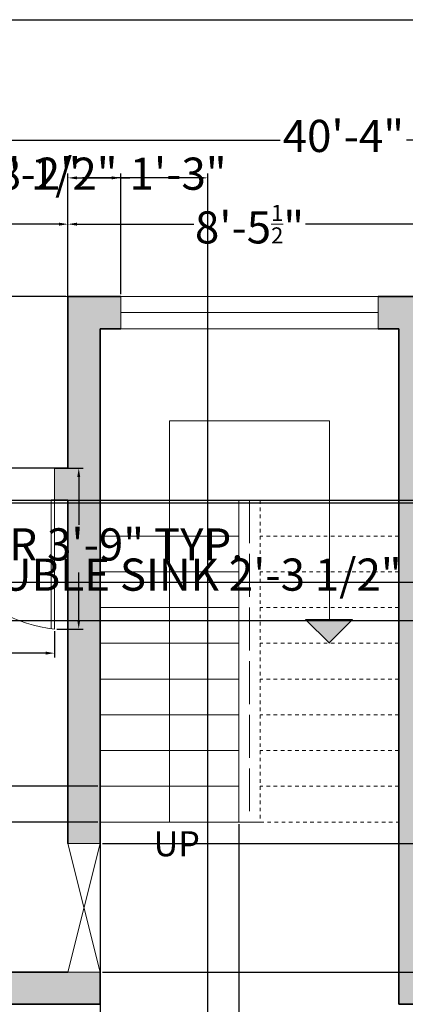
# Model space of a CAD drawing. Units: inches. Extents: x 1942 to 2601, y 2026 to 2623.
# Tile 3 of 5: x 2151 to 2259, y 2348 to 2623. Entities that reach past the tile are written whole.
import ezdxf

# ---------------------------------------------------------------- set-up
doc = ezdxf.new("R2010")
doc.units = ezdxf.units.IN
doc.linetypes.add('ACAD_ISO02W100', pattern=[15, 12, -3])
doc.linetypes.add('JIS_02_1.0', pattern=[2, 1, -1])
for name, color, linetype, lineweight in [('A-ANNO-DIMS', 2, 'Continuous', 18), ('A-ANNO-SYMB', 7, 'Continuous', 18), ('A-ANNO-TEXT', 7, 'Continuous', 18), ('A-ANNO-TTLB', 7, 'Continuous', 25), ('A-DOOR', 4, 'Continuous', 18), ('A-FLOR-OTLN', 8, 'ACAD_ISO02W100', 13), ('A-FLOR-STRS', 7, 'Continuous', 18), ('A-FLOR-STRS-CL', 8, 'ACAD_ISO02W100', 13), ('A-FLOR-STRS-HIDN', 7, 'JIS_02_1.0', 13), ('A-GLAZ', 2, 'Continuous', 18), ('A-WALL', 7, 'Continuous', 35), ('A-WALL-PATT', 7, 'Continuous', 13)]:
    doc.layers.add(name, color=color, linetype=linetype, lineweight=lineweight)
doc.styles.get("Standard").update_dxf_attribs({"font": 'arial.ttf'})
doc.dimstyles.new('ISO-25', dxfattribs={"dimtxt": 9, "dimasz": 2.5, "dimexe": 1.25, "dimexo": 0.625, "dimgap": 2, "dimtad": 0, "dimtih": 1, "dimtoh": 1, "dimdec": 1, "dimlunit": 4, "dimtxsty": 'Standard', "dimcen": 2.5, "dimadec": 0, "dimazin": 0, "dimtfac": 0.5, "dimtdec": 1, "dimtmove": 0, "dimatfit": 3, "dimfxl": 1, "dimarcsym": 0})

# ---------------------------------------------------------------- blocks, each defined once
blk = doc.blocks.new('*D11')
at = {"layer": 'A-ANNO-DIMS', "color": 0, "lineweight": -2, "transparency": 16777216}
for p, q in [((2164.82, 2546.54), (2164.82, 2567.42)), ((2266.32, 2546.54), (2266.32, 2567.42)), ((2167.32, 2566.17), (2199.96, 2566.17)), ((2263.82, 2566.17), (2231.18, 2566.17))]:
    blk.add_line(p, q, dxfattribs=at)
at = {"layer": 'A-ANNO-DIMS', "color": 0, "transparency": 16777216}
for points in [[(2167.32, 2566.58), (2167.32, 2565.75), (2164.82, 2566.17)], [(2263.82, 2566.58), (2263.82, 2565.75), (2266.32, 2566.17)]]:
    blk.add_solid(points, dxfattribs=at)
at = {"layer": 'Defpoints', "color": 0, "transparency": 16777216}
for p in [(2266.32, 2566.17), (2164.82, 2545.91), (2266.32, 2545.91)]:
    blk.add_point(p, dxfattribs=at)
at = {"layer": 'A-ANNO-DIMS', "color": 0, "transparency": 16777216, "insert": (2215.57, 2566.17), "char_height": 9, "attachment_point": 5}
blk.add_mtext('8\'-5{\\H0.5x;\\S1/2;}"', dxfattribs=at)
blk = doc.blocks.new('*D12')
at = {"layer": 'A-ANNO-DIMS', "color": 0, "lineweight": -2, "transparency": 16777216}
for p, q in [((1999.82, 2498.54), (1999.82, 2567.42)), ((2164.82, 2498.54), (2164.82, 2567.42)), ((2002.32, 2566.17), (2065.28, 2566.17)), ((2162.32, 2566.17), (2099.35, 2566.17))]:
    blk.add_line(p, q, dxfattribs=at)
at = {"layer": 'A-ANNO-DIMS', "color": 0, "transparency": 16777216}
for points in [[(2002.32, 2566.58), (2002.32, 2565.75), (1999.82, 2566.17)], [(2162.32, 2566.58), (2162.32, 2565.75), (2164.82, 2566.17)]]:
    blk.add_solid(points, dxfattribs=at)
at = {"layer": 'Defpoints', "color": 0, "transparency": 16777216}
for p in [(2164.82, 2566.17), (1999.82, 2497.91), (2164.82, 2497.91)]:
    blk.add_point(p, dxfattribs=at)
at = {"layer": 'A-ANNO-DIMS', "color": 0, "transparency": 16777216, "insert": (2082.32, 2566.17), "char_height": 9, "attachment_point": 5}
blk.add_mtext('13\'-9"', dxfattribs=at)
blk = doc.blocks.new('*D14')
at = {"layer": 'A-ANNO-DIMS', "color": 0, "lineweight": -2, "transparency": 16777216}
for p, q in [((1999.82, 2498.54), (1999.82, 2590.94)), ((2002.32, 2589.69), (2224.18, 2589.69)), ((2481.32, 2589.69), (2259.46, 2589.69)), ((2483.82, 2498.54), (2483.82, 2590.94))]:
    blk.add_line(p, q, dxfattribs=at)
at = {"layer": 'A-ANNO-DIMS', "color": 0, "transparency": 16777216}
for points in [[(2002.32, 2590.1), (2002.32, 2589.27), (1999.82, 2589.69)], [(2481.32, 2590.1), (2481.32, 2589.27), (2483.82, 2589.69)]]:
    blk.add_solid(points, dxfattribs=at)
at = {"layer": 'Defpoints', "color": 0, "transparency": 16777216}
for p in [(2483.82, 2589.69), (1999.82, 2497.91), (2483.82, 2497.91)]:
    blk.add_point(p, dxfattribs=at)
at = {"layer": 'A-ANNO-DIMS', "color": 0, "transparency": 16777216, "insert": (2241.82, 2589.69), "char_height": 9, "attachment_point": 5}
blk.add_mtext('40\'-4"', dxfattribs=at)
blk = doc.blocks.new('*D16')
at = {"layer": 'A-ANNO-DIMS', "color": 0, "lineweight": -2, "transparency": 16777216}
for p, q in [((2164.19, 2545.91), (1979.76, 2545.91)), ((1981.01, 2543.41), (1981.01, 2528.41)), ((1981.01, 2500.41), (1981.01, 2515.41)), ((2164.19, 2497.91), (1979.76, 2497.91))]:
    blk.add_line(p, q, dxfattribs=at)
at = {"layer": 'A-ANNO-DIMS', "color": 0, "transparency": 16777216}
for points in [[(1980.59, 2543.41), (1981.43, 2543.41), (1981.01, 2545.91)], [(1980.59, 2500.41), (1981.43, 2500.41), (1981.01, 2497.91)]]:
    blk.add_solid(points, dxfattribs=at)
at = {"layer": 'Defpoints', "color": 0, "transparency": 16777216}
for p in [(2164.82, 2545.91), (1981.01, 2497.91), (2164.82, 2497.91)]:
    blk.add_point(p, dxfattribs=at)
at = {"layer": 'A-ANNO-DIMS', "color": 0, "transparency": 16777216, "insert": (1981.01, 2521.91), "char_height": 9, "attachment_point": 5}
blk.add_mtext("4'", dxfattribs=at)
blk = doc.blocks.new('WIN-72IN')
for p, q in [((0, 0), (0, 9)), ((0, 9), (72, 9)), ((72, 0), (72, 9)), ((0, 4.5), (72, 4.5)), ((0, 0), (72, 0))]:
    blk.add_line(p, q)
blk = doc.blocks.new('DOOR-SINGLE-36IN')
for p, q in [((0, 9), (0, 45)), ((1, 9), (1, 44.88)), ((0, 0), (0, 9)), ((36, 0), (36, 9))]:
    blk.add_line(p, q)
blk.add_arc((-4.5, 4.5), 40.75, 353.6598, 83.6598)
blk = doc.blocks.new('*D35')
at = {"layer": 'A-ANNO-DIMS', "color": 0, "lineweight": -2, "transparency": 16777216}
for p, q in [((2161.7, 2497.91), (2169.07, 2497.91)), ((2167.82, 2495.41), (2167.82, 2482.07)), ((2167.82, 2455.41), (2167.82, 2468.75)), ((2161.7, 2452.91), (2169.07, 2452.91))]:
    blk.add_line(p, q, dxfattribs=at)
at = {"layer": 'A-ANNO-DIMS', "color": 0, "transparency": 16777216}
for points in [[(2167.41, 2495.41), (2168.24, 2495.41), (2167.82, 2497.91)], [(2167.41, 2455.41), (2168.24, 2455.41), (2167.82, 2452.91)]]:
    blk.add_solid(points, dxfattribs=at)
at = {"layer": 'Defpoints', "color": 0, "transparency": 16777216}
for p in [(2161.07, 2497.91), (2161.07, 2452.91), (2167.82, 2452.91)]:
    blk.add_point(p, dxfattribs=at)
at = {"layer": 'A-ANNO-DIMS', "color": 0, "transparency": 16777216, "insert": (2167.82, 2475.41), "char_height": 9, "attachment_point": 5}
blk.add_mtext('DOOR 3\'-9" TYP.', dxfattribs=at)
blk = doc.blocks.new('*D36')
at = {"layer": 'A-ANNO-DIMS', "color": 0, "lineweight": -2, "transparency": 16777216}
for p, q in [((2122.59, 2452.29), (2122.59, 2444.91)), ((2161.07, 2452.29), (2161.07, 2444.91)), ((2122.59, 2446.16), (2120.09, 2446.16)), ((2158.57, 2446.16), (2125.09, 2446.16))]:
    blk.add_line(p, q, dxfattribs=at)
at = {"layer": 'A-ANNO-DIMS', "color": 0, "transparency": 16777216}
for points in [[(2125.09, 2446.58), (2125.09, 2445.75), (2122.59, 2446.16)], [(2158.57, 2446.58), (2158.57, 2445.75), (2161.07, 2446.16)]]:
    blk.add_solid(points, dxfattribs=at)
at = {"layer": 'Defpoints', "color": 0, "transparency": 16777216}
for p in [(2122.59, 2452.91), (2161.07, 2452.91), (2122.59, 2446.16)]:
    blk.add_point(p, dxfattribs=at)
at = {"layer": 'A-ANNO-DIMS', "color": 0, "transparency": 16777216, "insert": (2080.18, 2446.16), "char_height": 9, "attachment_point": 5}
blk.add_mtext('3\'-2 1/2" TYP.', dxfattribs=at)
blk = doc.blocks.new('*D49')
at = {"layer": 'A-ANNO-DIMS', "color": 0, "lineweight": -2, "transparency": 16777216}
for p, q in [((2094.95, 2470.45), (2094.95, 2465.71)), ((2122.41, 2470.45), (2122.41, 2465.71)), ((2097.45, 2466.96), (2119.91, 2466.96)), ((2122.41, 2466.96), (2124.91, 2466.96))]:
    blk.add_line(p, q, dxfattribs=at)
at = {"layer": 'A-ANNO-DIMS', "color": 0, "transparency": 16777216}
for points in [[(2097.45, 2467.38), (2097.45, 2466.54), (2094.95, 2466.96)], [(2119.91, 2467.38), (2119.91, 2466.54), (2122.41, 2466.96)]]:
    blk.add_solid(points, dxfattribs=at)
at = {"layer": 'Defpoints', "color": 0, "transparency": 16777216}
for p in [(2094.95, 2471.08), (2122.41, 2471.08), (2122.41, 2466.96)]:
    blk.add_point(p, dxfattribs=at)
at = {"layer": 'A-ANNO-DIMS', "color": 0, "transparency": 16777216, "insert": (2193.15, 2466.96), "char_height": 9, "attachment_point": 5}
blk.add_mtext('DOUBLE SINK 2\'-3 1/2"', dxfattribs=at)
blk = doc.blocks.new('*D55')
at = {"layer": 'A-ANNO-DIMS', "color": 0, "lineweight": -2, "transparency": 16777216}
for p, q in [((2114.04, 2579.12), (2111.54, 2579.12)), ((2116.54, 2498.54), (2116.54, 2580.37)), ((2116.54, 2579.12), (2125.07, 2579.12)), ((2125.07, 2498.54), (2125.07, 2580.37)), ((2127.57, 2579.12), (2130.07, 2579.12))]:
    blk.add_line(p, q, dxfattribs=at)
at = {"layer": 'A-ANNO-DIMS', "color": 0, "transparency": 16777216}
for points in [[(2114.04, 2579.54), (2114.04, 2578.7), (2116.54, 2579.12)], [(2127.57, 2579.54), (2127.57, 2578.7), (2125.07, 2579.12)]]:
    blk.add_solid(points, dxfattribs=at)
at = {"layer": 'Defpoints', "color": 0, "transparency": 16777216}
for p in [(2125.07, 2579.12), (2116.54, 2497.91), (2125.07, 2497.91)]:
    blk.add_point(p, dxfattribs=at)
at = {"layer": 'A-ANNO-DIMS', "color": 0, "transparency": 16777216, "insert": (2154.52, 2579.12), "char_height": 9, "attachment_point": 5}
blk.add_mtext('0\'-8 1/2"', dxfattribs=at)
blk = doc.blocks.new('*D57')
at = {"layer": 'A-ANNO-DIMS', "color": 0, "lineweight": -2, "transparency": 16777216}
for p, q in [((2164.82, 2546.54), (2164.82, 2580.37)), ((2167.32, 2579.12), (2177.07, 2579.12)), ((2179.57, 2546.54), (2179.57, 2580.37)), ((2179.57, 2579.12), (2182.07, 2579.12))]:
    blk.add_line(p, q, dxfattribs=at)
at = {"layer": 'A-ANNO-DIMS', "color": 0, "transparency": 16777216}
for points in [[(2167.32, 2579.54), (2167.32, 2578.7), (2164.82, 2579.12)], [(2177.07, 2579.54), (2177.07, 2578.7), (2179.57, 2579.12)]]:
    blk.add_solid(points, dxfattribs=at)
at = {"layer": 'Defpoints', "color": 0, "transparency": 16777216}
for p in [(2179.57, 2579.12), (2164.82, 2545.91), (2179.57, 2545.91)]:
    blk.add_point(p, dxfattribs=at)
at = {"layer": 'A-ANNO-DIMS', "color": 0, "transparency": 16777216, "insert": (2195.61, 2579.12), "char_height": 9, "attachment_point": 5}
blk.add_mtext('1\'-3"', dxfattribs=at)
blk = doc.blocks.new('*D66')
at = {"layer": 'A-ANNO-DIMS', "color": 0, "lineweight": -2, "transparency": 16777216}
for p, q in [((2105.82, 2167.54), (2105.82, 2580.37)), ((2108.32, 2579.12), (2140.9, 2579.12)), ((2201.42, 2579.12), (2168.84, 2579.12)), ((2203.92, 2167.54), (2203.92, 2580.37))]:
    blk.add_line(p, q, dxfattribs=at)
at = {"layer": 'A-ANNO-DIMS', "color": 0, "transparency": 16777216}
for points in [[(2108.32, 2579.54), (2108.32, 2578.7), (2105.82, 2579.12)], [(2201.42, 2579.54), (2201.42, 2578.7), (2203.92, 2579.12)]]:
    blk.add_solid(points, dxfattribs=at)
at = {"layer": 'Defpoints', "color": 0, "transparency": 16777216}
for p in [(2203.92, 2579.12), (2105.82, 2166.91), (2203.92, 2166.91)]:
    blk.add_point(p, dxfattribs=at)
at = {"layer": 'A-ANNO-DIMS', "color": 0, "transparency": 16777216, "insert": (2154.87, 2579.12), "char_height": 9, "attachment_point": 5}
blk.add_mtext('8\'-2"', dxfattribs=at)
blk = doc.blocks.new('*D70')
at = {"layer": 'A-ANNO-DIMS', "color": 0, "lineweight": -2, "transparency": 16777216}
for p, q in [((1968.82, 2408.91), (1968.82, 2411.41)), ((1968.82, 2411.41), (1971.32, 2411.41)), ((2173.19, 2408.91), (1967.57, 2408.91)), ((1968.82, 2401.41), (1968.82, 2406.41)), ((2173.19, 2398.91), (1967.57, 2398.91))]:
    blk.add_line(p, q, dxfattribs=at)
at = {"layer": 'A-ANNO-DIMS', "color": 0, "transparency": 16777216}
for points in [[(1968.4, 2406.41), (1969.24, 2406.41), (1968.82, 2408.91)], [(1968.4, 2401.41), (1969.24, 2401.41), (1968.82, 2398.91)]]:
    blk.add_solid(points, dxfattribs=at)
at = {"layer": 'Defpoints', "color": 0, "transparency": 16777216}
for p in [(1968.82, 2408.91), (2173.82, 2408.91), (2173.82, 2398.91)]:
    blk.add_point(p, dxfattribs=at)
at = {"layer": 'A-ANNO-DIMS', "color": 0, "transparency": 16777216, "insert": (1988.78, 2411.41), "char_height": 9, "attachment_point": 5}
blk.add_mtext('0\'-10"', dxfattribs=at)
blk = doc.blocks.new('*D71')
at = {"layer": 'A-ANNO-DIMS', "color": 0, "lineweight": -2, "transparency": 16777216}
for p, q in [((2173.82, 2398.29), (2173.82, 2041.66)), ((2212.57, 2398.29), (2212.57, 2041.66)), ((2176.32, 2042.91), (2179.24, 2042.91)), ((2210.07, 2042.91), (2207.15, 2042.91))]:
    blk.add_line(p, q, dxfattribs=at)
at = {"layer": 'A-ANNO-DIMS', "color": 0, "transparency": 16777216}
for points in [[(2176.32, 2043.33), (2176.32, 2042.5), (2173.82, 2042.91)], [(2210.07, 2043.33), (2210.07, 2042.5), (2212.57, 2042.91)]]:
    blk.add_solid(points, dxfattribs=at)
at = {"layer": 'Defpoints', "color": 0, "transparency": 16777216}
for p in [(2173.82, 2398.91), (2212.57, 2398.91), (2212.57, 2042.91)]:
    blk.add_point(p, dxfattribs=at)
at = {"layer": 'A-ANNO-DIMS', "color": 0, "transparency": 16777216, "insert": (2193.19, 2042.91), "char_height": 9, "attachment_point": 5}
blk.add_mtext('3\'-3"', dxfattribs=at)
blk = doc.blocks.new('*D72')
at = {"layer": 'A-ANNO-DIMS', "color": 0, "lineweight": -2, "transparency": 16777216}
for p, q in [((2174.44, 2392.91), (2516.07, 2392.91)), ((2514.82, 2390.41), (2514.82, 2381.51)), ((2514.82, 2359.41), (2514.82, 2368.32)), ((2174.44, 2356.91), (2516.07, 2356.91))]:
    blk.add_line(p, q, dxfattribs=at)
at = {"layer": 'A-ANNO-DIMS', "color": 0, "transparency": 16777216}
for points in [[(2514.4, 2390.41), (2515.24, 2390.41), (2514.82, 2392.91)], [(2514.4, 2359.41), (2515.24, 2359.41), (2514.82, 2356.91)]]:
    blk.add_solid(points, dxfattribs=at)
at = {"layer": 'Defpoints', "color": 0, "transparency": 16777216}
for p in [(2173.82, 2392.91), (2514.82, 2392.91), (2173.82, 2356.91)]:
    blk.add_point(p, dxfattribs=at)
at = {"layer": 'A-ANNO-DIMS', "color": 0, "transparency": 16777216, "insert": (2514.82, 2374.91), "char_height": 9, "attachment_point": 5}
blk.add_mtext('3\'-0"', dxfattribs=at)
blk = doc.blocks.new('*D74')
at = {"layer": 'A-ANNO-DIMS', "color": 0, "lineweight": -2, "transparency": 16777216}
for p, q in [((2009.44, 2488.91), (2516.07, 2488.91)), ((2514.82, 2486.41), (2514.82, 2484)), ((2514.82, 2468.55), (2514.82, 2470.96)), ((2029.44, 2466.05), (2516.07, 2466.05))]:
    blk.add_line(p, q, dxfattribs=at)
at = {"layer": 'A-ANNO-DIMS', "color": 0, "transparency": 16777216}
for points in [[(2514.4, 2486.41), (2515.24, 2486.41), (2514.82, 2488.91)], [(2514.4, 2468.55), (2515.24, 2468.55), (2514.82, 2466.05)]]:
    blk.add_solid(points, dxfattribs=at)
at = {"layer": 'Defpoints', "color": 0, "transparency": 16777216}
for p in [(2008.82, 2488.91), (2514.82, 2488.91), (2028.82, 2466.05)]:
    blk.add_point(p, dxfattribs=at)
at = {"layer": 'A-ANNO-DIMS', "color": 0, "transparency": 16777216, "insert": (2514.82, 2477.48), "char_height": 9, "attachment_point": 5}
blk.add_mtext('1\'-11"', dxfattribs=at)
blk = doc.blocks.new('*D76')
at = {"layer": 'A-ANNO-DIMS', "color": 0, "lineweight": -2, "transparency": 16777216}
for p, q in [((2295.53, 2488.12), (1967.57, 2488.12)), ((1968.82, 2485.62), (1968.82, 2478.23)), ((1968.82, 2457.66), (1968.82, 2465.04)), ((2295, 2455.16), (1967.57, 2455.16))]:
    blk.add_line(p, q, dxfattribs=at)
at = {"layer": 'A-ANNO-DIMS', "color": 0, "transparency": 16777216}
for points in [[(1968.4, 2485.62), (1969.24, 2485.62), (1968.82, 2488.12)], [(1968.4, 2457.66), (1969.24, 2457.66), (1968.82, 2455.16)]]:
    blk.add_solid(points, dxfattribs=at)
at = {"layer": 'Defpoints', "color": 0, "transparency": 16777216}
for p in [(1968.82, 2488.12), (2296.15, 2488.12), (2295.63, 2455.16)]:
    blk.add_point(p, dxfattribs=at)
at = {"layer": 'A-ANNO-DIMS', "color": 0, "transparency": 16777216, "insert": (1968.82, 2471.64), "char_height": 9, "attachment_point": 5}
blk.add_mtext('2\'-9"', dxfattribs=at)

msp = doc.modelspace()

# ---------------------------------------------------------------- hatches: boundary and pattern name
at = {"layer": 'A-ANNO-SYMB'}
h = msp.add_hatch(color=256, dxfattribs=at)
h.dxf.hatch_style = 1
h.paths.add_polyline_path([(2244.34, 2455.58), (2231.24, 2455.58), (2237.83, 2449.02)])
at = {"layer": 'A-WALL-PATT'}
h = msp.add_hatch(color=256, dxfattribs=at)
h.dxf.hatch_style = 1
h.paths.add_polyline_path([(2056.54, 2497.91), (1999.82, 2497.91), (1999.82, 2347.91), (2008.82, 2347.91), (2028.82, 2347.91), (2028.82, 2356.91), (2008.82, 2356.91), (2008.82, 2488.91), (2056.54, 2488.91)])
h.paths.add_polyline_path([(2173.82, 2356.91), (2164.82, 2356.91), (2076.82, 2356.91), (2076.82, 2347.91), (2096.82, 2347.91), (2105.82, 2347.91), (2164.82, 2347.91), (2173.82, 2347.91)])
h.paths.add_polyline_path([(2173.82, 2488.91), (2173.82, 2497.91), (2173.82, 2536.91), (2179.57, 2536.91), (2179.57, 2545.91), (2173.82, 2545.91), (2164.82, 2545.91), (2164.82, 2497.91), (2161.07, 2497.91), (2161.07, 2488.91), (2164.82, 2488.91), (2164.82, 2392.91), (2173.82, 2392.91)])
h.paths.add_polyline_path([(2125.07, 2497.91), (2116.54, 2497.91), (2116.54, 2488.91), (2125.07, 2488.91, -0.055385)])
h.paths.add_polyline_path([(2266.32, 2545.91), (2257.32, 2545.91), (2251.57, 2545.91), (2251.57, 2536.91), (2257.32, 2536.91), (2257.32, 2497.91), (2257.32, 2488.91), (2257.32, 2347.91), (2318.82, 2347.91), (2342.82, 2347.91), (2342.82, 2356.91), (2318.82, 2356.91), (2318.82, 2386.91), (2314.32, 2386.91), (2314.32, 2356.91), (2266.32, 2356.91), (2266.32, 2410.91), (2289.34, 2410.91, -0.055385), (2289.34, 2416.91), (2266.32, 2416.91), (2266.32, 2488.91), (2278.32, 2488.91), (2278.32, 2497.91), (2266.32, 2497.91)])
h.paths.add_polyline_path([(2360.82, 2497.91), (2314.32, 2497.91), (2314.32, 2488.91), (2314.32, 2416.91), (2314.32, 2410.91), (2318.82, 2410.91), (2318.82, 2488.91), (2360.82, 2488.91)])
h.paths.add_polyline_path([(2483.82, 2497.91), (2432.82, 2497.91), (2432.82, 2488.91), (2474.82, 2488.91), (2474.82, 2458.91), (2483.82, 2458.91)])
h.paths.add_polyline_path([(2483.82, 2386.91), (2474.82, 2386.91), (2474.82, 2356.91), (2378.82, 2356.91, -0.055385), (2378.82, 2347.91), (2386.82, 2347.91), (2386.82, 2299.91), (2386.82, 2293.91), (2394.45, 2293.91), (2394.45, 2299.91), (2392.82, 2299.91), (2392.82, 2347.91), (2474.82, 2347.91), (2474.82, 2341.91), (2483.82, 2341.91)])
h.paths.add_polyline_path([(2483.82, 2305.91), (2474.82, 2305.91), (2474.82, 2299.91), (2418.45, 2299.91, -0.055385), (2418.45, 2293.91), (2420.82, 2293.91), (2420.82, 2285.08, -0.055385), (2426.82, 2285.08), (2426.82, 2293.91), (2474.82, 2293.91), (2474.82, 2288.91), (2483.82, 2288.91)])

# ---------------------------------------------------------------- linework, layer by layer
at = {"layer": 'A-ANNO-SYMB'}
for p, q in [((2193.19, 2398.91), (2193.19, 2511.15)), ((2193.19, 2511.15), (2237.94, 2511.15)), ((2237.94, 2455.58), (2237.94, 2511.15)), ((2237.94, 2448.91), (2231.24, 2455.58)), ((2231.24, 2455.58), (2244.34, 2455.58)), ((2244.34, 2455.58), (2237.83, 2449.02)), ((2237.94, 2448.91), (2237.94, 2449.14))]:
    msp.add_line(p, q, dxfattribs=at)
at = {"layer": 'A-ANNO-TTLB'}
msp.add_lwpolyline([(1941.67, 2623.37), (2601.3, 2623.37), (2601.3, 2026.31), (1941.67, 2026.31)], close=True, dxfattribs=at)
at = {"layer": 'A-DOOR'}
for p, q in [((2164.82, 2392.91), (2173.82, 2392.91)), ((2164.82, 2392.91), (2173.82, 2356.91)), ((2173.82, 2392.91), (2164.82, 2356.91)), ((2164.82, 2356.91), (2173.82, 2356.91))]:
    msp.add_line(p, q, dxfattribs=at)
at = {"layer": 'A-FLOR-OTLN'}
msp.add_line((2164.82, 2545.91), (1999.82, 2545.91), dxfattribs=at)
at = {"layer": 'A-FLOR-STRS'}
for p, q in [((2218.57, 2488.91), (2173.82, 2488.91)), ((2212.57, 2488.91), (2212.57, 2398.91)), ((2212.57, 2478.91), (2173.82, 2478.91)), ((2212.57, 2468.91), (2173.82, 2468.91)), ((2212.57, 2458.91), (2173.82, 2458.91)), ((2212.57, 2448.91), (2173.82, 2448.91)), ((2212.57, 2438.91), (2173.82, 2438.91)), ((2212.57, 2428.91), (2173.82, 2428.91)), ((2212.57, 2418.91), (2173.82, 2418.91)), ((2212.57, 2408.91), (2173.82, 2408.91)), ((2218.57, 2398.91), (2173.82, 2398.91)), ((2212.57, 2398.91), (2173.82, 2398.91))]:
    msp.add_line(p, q, dxfattribs=at)
at = {"layer": 'A-FLOR-STRS-CL'}
msp.add_line((2215.57, 2488.91), (2215.57, 2398.91), dxfattribs=at)
at = {"layer": 'A-FLOR-STRS-HIDN'}
for p, q in [((2218.57, 2488.91), (2218.57, 2398.91)), ((2218.57, 2488.91), (2257.32, 2488.91)), ((2257.32, 2478.91), (2218.57, 2478.91)), ((2257.32, 2468.91), (2218.57, 2468.91)), ((2257.32, 2458.91), (2218.57, 2458.91)), ((2257.32, 2448.91), (2218.57, 2448.91)), ((2257.32, 2438.91), (2218.57, 2438.91)), ((2257.32, 2428.91), (2218.57, 2428.91)), ((2257.32, 2418.91), (2218.57, 2418.91)), ((2257.32, 2408.91), (2218.57, 2408.91)), ((2218.57, 2398.91), (2257.32, 2398.91))]:
    msp.add_line(p, q, dxfattribs=at)
at = {"layer": 'A-WALL'}
for p, q in [((2164.82, 2497.91), (2164.82, 2545.91)), ((2173.82, 2545.91), (2164.82, 2545.91)), ((2164.82, 2545.91), (2164.82, 2497.91)), ((2173.82, 2545.91), (2179.57, 2545.91)), ((2251.57, 2545.91), (2257.32, 2545.91)), ((2257.32, 2545.91), (2266.32, 2545.91)), ((2173.82, 2536.91), (2179.57, 2536.91)), ((2173.82, 2497.91), (2173.82, 2536.91)), ((2251.57, 2536.91), (2257.32, 2536.91)), ((2257.32, 2497.91), (2257.32, 2536.91)), ((2161.07, 2497.91), (2164.82, 2497.91)), ((2173.82, 2488.91), (2173.82, 2497.91)), ((2257.32, 2488.91), (2257.32, 2497.91)), ((2160.07, 2488.91), (2164.82, 2488.91)), ((2164.82, 2392.91), (2164.82, 2488.91)), ((2173.82, 2392.91), (2173.82, 2488.91)), ((2257.32, 2488.91), (2257.32, 2347.91)), ((2076.82, 2356.91), (2164.82, 2356.91)), ((2173.82, 2347.91), (2173.82, 2356.91)), ((2105.82, 2347.91), (2164.82, 2347.91)), ((2164.82, 2347.91), (2173.82, 2347.91)), ((2318.82, 2347.91), (2257.32, 2347.91))]:
    msp.add_line(p, q, dxfattribs=at)

# ---------------------------------------------------------------- block references
at = {"layer": 'A-DOOR', "rotation": 180}
msp.add_blockref('DOOR-SINGLE-36IN', (2161.07, 2497.91), dxfattribs=at)
at = {"layer": 'A-GLAZ'}
msp.add_blockref('WIN-72IN', (2179.57, 2536.91), dxfattribs=at)

# ---------------------------------------------------------------- texts
at = {"layer": 'A-ANNO-TEXT', "insert": (2188.76, 2396.33), "char_height": 7, "attachment_point": 1}
msp.add_mtext_dynamic_manual_height_columns('UP', width=11.3397, gutter_width=12.5, heights=[0], dxfattribs=at)

# ---------------------------------------------------------------- dimensions: what is measured, and where the dimension line sits
at = {"layer": 'A-ANNO-DIMS'}
for base, p1, p2, override, picture, middle in [((2483.82, 2589.69), (1999.82, 2497.91), (2483.82, 2497.91), {"dimclrd": 0, "dimclre": 0, "dimclrt": 0}, '*D14', (2241.82, 2589.69)), ((2125.07, 2579.12), (2116.54, 2497.91), (2125.07, 2497.91), {"dimdec": 1, "dimlfac": 1, "dimrnd": 0, "dimzin": 1, "dimdsep": 46, "dimlunit": 4, "dimfrac": 2}, '*D55', (2154.52, 2579.12)), ((2203.92, 2579.12), (2105.82, 2166.91), (2203.92, 2166.91), {"dimdec": 1, "dimlfac": 1, "dimrnd": 0, "dimzin": 1, "dimdsep": 46, "dimlunit": 4, "dimfrac": 2}, '*D66', (2154.87, 2579.12)), ((2179.569724, 2579.121409), (2164.819724, 2545.91449), (2179.569724, 2545.91449), {"dimdec": 1, "dimlfac": 1, "dimrnd": 0, "dimzin": 1, "dimdsep": 46, "dimlunit": 4, "dimfrac": 2}, '*D57', (2195.60826425, 2579.121409)), ((2164.82, 2566.17), (1999.82, 2497.91), (2164.82, 2497.91), {"dimclrd": 0, "dimclre": 0, "dimclrt": 0}, '*D12', (2082.32, 2566.17)), ((2266.32, 2566.17), (2164.82, 2545.91), (2266.32, 2545.91), {"dimclrd": 0, "dimclre": 0, "dimclrt": 0}, '*D11', (2215.57, 2566.17)), ((2212.569724, 2042.91449), (2173.819724, 2398.91449), (2212.569724, 2398.91449), {"dimdec": 1, "dimlfac": 1, "dimrnd": 0, "dimzin": 1, "dimdsep": 46, "dimlunit": 4, "dimfrac": 2}, '*D71', (2193.194724, 2042.91449))]:
    dim = msp.add_linear_dim(base=base, p1=p1, p2=p2, dimstyle='ISO-25', override=override, dxfattribs=at)
    dim.commit()
    dim.dimension.update_dxf_attribs({"geometry": picture, "text_midpoint": middle})
for base, p1, p2, override, picture, middle in [((1981.01, 2497.91), (2164.82, 2545.91), (2164.82, 2497.91), {"dimclrd": 0, "dimclre": 0, "dimclrt": 0}, '*D16', (1981.01, 2521.91)), ((1968.82, 2488.12), (2295.63, 2455.16), (2296.15, 2488.12), {"dimdec": 1, "dimlfac": 1, "dimrnd": 0, "dimzin": 1, "dimdsep": 46, "dimlunit": 4, "dimfrac": 2}, '*D76', (1968.82, 2471.64)), ((2514.82, 2488.91), (2028.82, 2466.05), (2008.82, 2488.91), {"dimdec": 1, "dimlfac": 1, "dimrnd": 0, "dimzin": 1, "dimdsep": 46, "dimlunit": 4, "dimfrac": 2}, '*D74', (2514.82, 2477.48)), ((1968.82, 2408.91), (2173.82, 2398.91), (2173.82, 2408.91), {"dimdec": 1, "dimlfac": 1, "dimrnd": 0, "dimzin": 1, "dimdsep": 46, "dimlunit": 4, "dimfrac": 2}, '*D70', (1988.78, 2411.41)), ((2514.82, 2392.91), (2173.82, 2356.91), (2173.82, 2392.91), {"dimdec": 1, "dimlfac": 1, "dimrnd": 0, "dimzin": 1, "dimdsep": 46, "dimlunit": 4, "dimfrac": 2}, '*D72', (2514.82, 2374.91))]:
    dim = msp.add_linear_dim(base=base, p1=p1, p2=p2, angle=90, dimstyle='ISO-25', override=override, dxfattribs=at)
    dim.commit()
    dim.dimension.update_dxf_attribs({"geometry": picture, "text_midpoint": middle})
for base, p1, p2, angle, text, picture, middle in [((2167.82, 2452.91), (2161.07, 2497.91), (2161.07, 2452.91), 270, 'DOOR <> TYP.', '*D35', (2167.82, 2475.41)), ((2122.59, 2446.16), (2161.07, 2452.91), (2122.59, 2452.91), 180, '<> TYP.', '*D36', (2080.18, 2446.16))]:
    dim = msp.add_linear_dim(base=base, p1=p1, p2=p2, angle=angle, text=text, dimstyle='ISO-25', override={"dimdec": 1, "dimlfac": 1, "dimrnd": 0, "dimzin": 1, "dimdsep": 46, "dimlunit": 4, "dimfrac": 2}, dxfattribs=at)
    dim.commit()
    dim.dimension.update_dxf_attribs({"geometry": picture, "text_midpoint": middle})
dim = msp.add_linear_dim(base=(2122.41, 2466.96), p1=(2094.95, 2471.08), p2=(2122.41, 2471.08), text='DOUBLE SINK <>', dimstyle='ISO-25', override={"dimdec": 1, "dimlfac": 1, "dimrnd": 0, "dimzin": 1, "dimdsep": 46, "dimlunit": 4, "dimfrac": 2}, dxfattribs=at)
dim.commit()
dim.dimension.update_dxf_attribs({"geometry": '*D49', "text_midpoint": (2193.15, 2466.96)})

doc.saveas('drawing.dxf')
